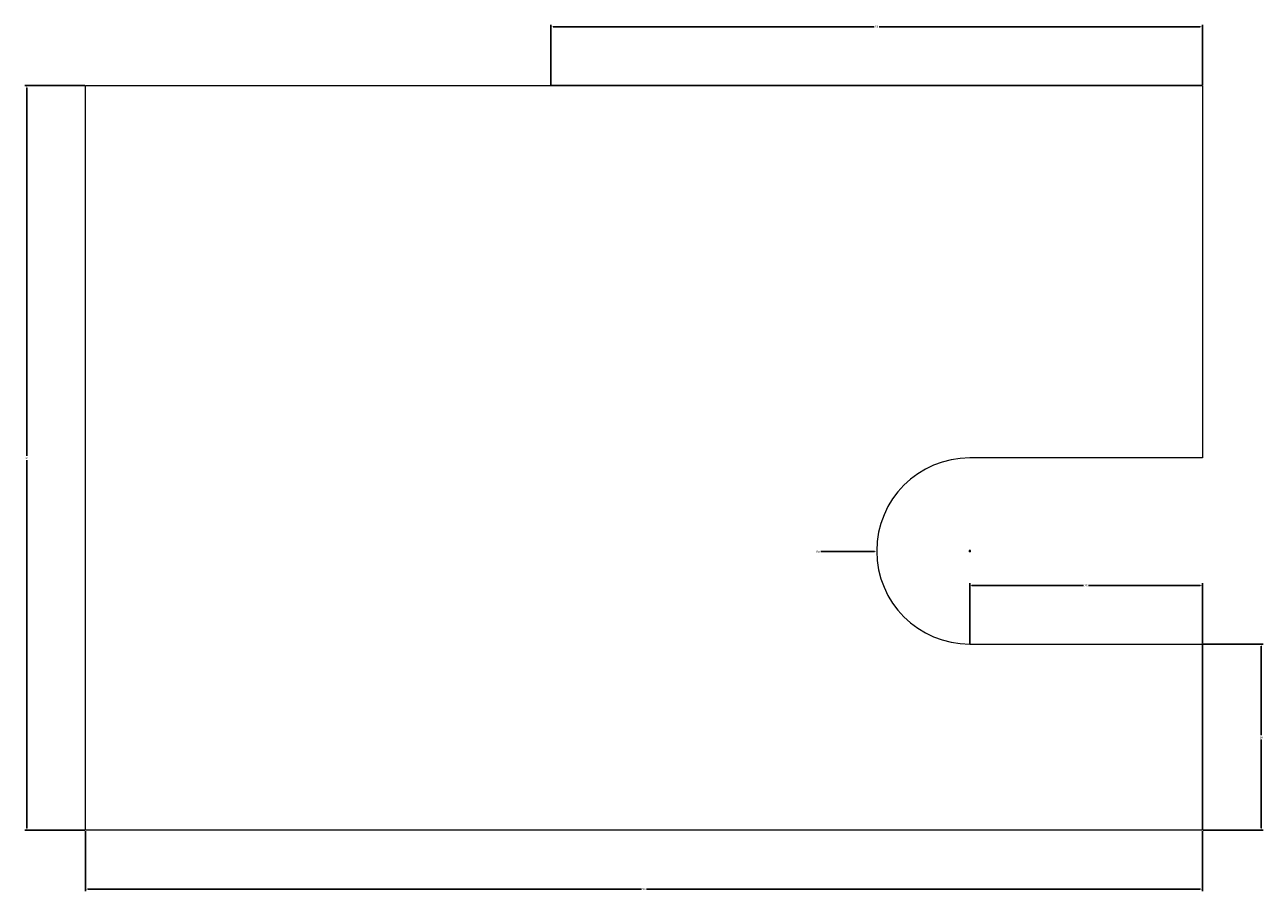
# Model space of a CAD drawing. Units: millimetres. Extents: x -4 to 2856, y -2 to 1373.
# Tile 3 of 3: x 2749 to 2856, y 1175 to 1249. Entities that reach past the tile are written whole.
import ezdxf

# ---------------------------------------------------------------- set-up
doc = ezdxf.new("R2010")
doc.units = ezdxf.units.MM
doc.layers.add('M-CONS', color=8, linetype='Continuous', lineweight=18)
doc.layers.add('M-DIMS', color=2, linetype='Continuous', lineweight=18)
doc.styles.get("Standard").update_dxf_attribs({"font": 'arial.ttf'})
doc.dimstyles.get("Standard").update_dxf_attribs({"dimtxt": 0.18, "dimasz": 0.18, "dimexe": 0.18, "dimexo": 0.0625, "dimgap": 0.09, "dimtad": 0, "dimtih": 1, "dimtoh": 1, "dimdec": 4, "dimzin": 0, "dimdsep": 46, "dimtxsty": 'Standard', "dimcen": 0.09, "dimadec": 0, "dimazin": 0, "dimtfac": 1, "dimtdec": 4, "dimtofl": 0, "dimtmove": 0, "dimatfit": 3, "dimfxl": 1, "dimtolj": 1, "dimtzin": 0, "dimarcsym": 0})

# ---------------------------------------------------------------- blocks, each defined once
blk = doc.blocks.new('*D1')
at = {"layer": 'Defpoints', "color": 0, "transparency": 16777216}
for p in [(2850.61, 1249.28), (2794.61, 1244.23), (2850.61, 1244.23)]:
    blk.add_point(p, dxfattribs=at)
at = {"layer": 'M-DIMS', "color": 0, "lineweight": -2, "transparency": 16777216}
for p, q in [((2794.61, 1244.29), (2794.61, 1249.46)), ((2794.79, 1249.28), (2822.39, 1249.28)), ((2850.43, 1249.28), (2822.83, 1249.28)), ((2850.61, 1244.29), (2850.61, 1249.46))]:
    blk.add_line(p, q, dxfattribs=at)
at = {"layer": 'M-DIMS', "color": 0, "transparency": 16777216}
for points in [[(2794.79, 1249.31), (2794.79, 1249.25), (2794.61, 1249.28)], [(2850.43, 1249.31), (2850.43, 1249.25), (2850.61, 1249.28)]]:
    blk.add_solid(points, dxfattribs=at)
at = {"layer": 'M-DIMS', "color": 0, "transparency": 16777216, "insert": (2822.61, 1249.28), "char_height": 0.18, "attachment_point": 5}
blk.add_mtext('\\A1;56', dxfattribs=at)
blk = doc.blocks.new('*D2')
at = {"layer": 'Defpoints', "color": 0, "transparency": 16777216}
for p in [(2754.61, 1180.23), (2850.61, 1180.23), (2850.61, 1175.18)]:
    blk.add_point(p, dxfattribs=at)
at = {"layer": 'M-DIMS', "color": 0, "lineweight": -2, "transparency": 16777216}
for p, q in [((2754.61, 1180.16), (2754.61, 1175)), ((2850.61, 1180.16), (2850.61, 1175)), ((2754.79, 1175.18), (2802.39, 1175.18)), ((2850.43, 1175.18), (2802.83, 1175.18))]:
    blk.add_line(p, q, dxfattribs=at)
at = {"layer": 'M-DIMS', "color": 0, "transparency": 16777216}
for points in [[(2754.79, 1175.21), (2754.79, 1175.15), (2754.61, 1175.18)], [(2850.43, 1175.21), (2850.43, 1175.15), (2850.61, 1175.18)]]:
    blk.add_solid(points, dxfattribs=at)
at = {"layer": 'M-DIMS', "color": 0, "transparency": 16777216, "insert": (2802.61, 1175.18), "char_height": 0.18, "attachment_point": 5}
blk.add_mtext('\\A1;96', dxfattribs=at)
blk = doc.blocks.new('*D3')
at = {"layer": 'Defpoints', "color": 0, "transparency": 16777216}
for p in [(2749.56, 1244.23), (2754.61, 1244.23), (2754.61, 1180.23)]:
    blk.add_point(p, dxfattribs=at)
at = {"layer": 'M-DIMS', "color": 0, "lineweight": -2, "transparency": 16777216}
for p, q in [((2754.54, 1244.23), (2749.38, 1244.23)), ((2749.56, 1244.05), (2749.56, 1212.41)), ((2749.56, 1180.41), (2749.56, 1212.04)), ((2754.54, 1180.23), (2749.38, 1180.23))]:
    blk.add_line(p, q, dxfattribs=at)
at = {"layer": 'M-DIMS', "color": 0, "transparency": 16777216}
for points in [[(2749.53, 1244.05), (2749.59, 1244.05), (2749.56, 1244.23)], [(2749.53, 1180.41), (2749.59, 1180.41), (2749.56, 1180.23)]]:
    blk.add_solid(points, dxfattribs=at)
at = {"layer": 'M-DIMS', "color": 0, "transparency": 16777216, "insert": (2749.56, 1212.23), "char_height": 0.18, "attachment_point": 5}
blk.add_mtext('\\A1;64', dxfattribs=at)
blk = doc.blocks.new('*D4')
at = {"layer": 'Defpoints', "color": 0, "transparency": 16777216}
for p in [(2850.61, 1201.28), (2830.61, 1196.23), (2850.61, 1196.23)]:
    blk.add_point(p, dxfattribs=at)
at = {"layer": 'M-DIMS', "color": 0, "lineweight": -2, "transparency": 16777216}
for p, q in [((2830.61, 1196.29), (2830.61, 1201.46)), ((2830.79, 1201.28), (2840.39, 1201.28)), ((2850.43, 1201.28), (2840.83, 1201.28)), ((2850.61, 1196.29), (2850.61, 1201.46))]:
    blk.add_line(p, q, dxfattribs=at)
at = {"layer": 'M-DIMS', "color": 0, "transparency": 16777216}
for points in [[(2830.79, 1201.31), (2830.79, 1201.25), (2830.61, 1201.28)], [(2850.43, 1201.31), (2850.43, 1201.25), (2850.61, 1201.28)]]:
    blk.add_solid(points, dxfattribs=at)
at = {"layer": 'M-DIMS', "color": 0, "transparency": 16777216, "insert": (2840.61, 1201.28), "char_height": 0.18, "attachment_point": 5}
blk.add_mtext('\\A1;20', dxfattribs=at)
blk = doc.blocks.new('*D5')
at = {"layer": 'Defpoints', "color": 0, "transparency": 16777216}
for p in [(2850.61, 1196.23), (2855.66, 1196.23), (2850.61, 1180.23)]:
    blk.add_point(p, dxfattribs=at)
at = {"layer": 'M-DIMS', "color": 0, "lineweight": -2, "transparency": 16777216}
for p, q in [((2850.67, 1196.23), (2855.84, 1196.23)), ((2855.66, 1196.05), (2855.66, 1188.41)), ((2855.66, 1180.41), (2855.66, 1188.04)), ((2850.67, 1180.23), (2855.84, 1180.23))]:
    blk.add_line(p, q, dxfattribs=at)
at = {"layer": 'M-DIMS', "color": 0, "transparency": 16777216}
for points in [[(2855.63, 1196.05), (2855.69, 1196.05), (2855.66, 1196.23)], [(2855.63, 1180.41), (2855.69, 1180.41), (2855.66, 1180.23)]]:
    blk.add_solid(points, dxfattribs=at)
at = {"layer": 'M-DIMS', "color": 0, "transparency": 16777216, "insert": (2855.66, 1188.23), "char_height": 0.18, "attachment_point": 5}
blk.add_mtext('\\A1;16', dxfattribs=at)
blk = doc.blocks.new('*D10')
at = {"layer": 'Defpoints', "color": 0, "transparency": 16777216}
for p in [(2822.61, 1204.2), (2830.61, 1204.23)]:
    blk.add_point(p, dxfattribs=at)
at = {"layer": 'M-DIMS', "color": 0, "lineweight": -2, "transparency": 16777216}
for p, q in [((2817.81, 1204.18), (2822.43, 1204.2)), ((2830.52, 1204.23), (2830.7, 1204.23)), ((2830.61, 1204.14), (2830.61, 1204.32))]:
    blk.add_line(p, q, dxfattribs=at)
at = {"layer": 'M-DIMS', "color": 0, "transparency": 16777216}
blk.add_solid([(2822.43, 1204.23), (2822.43, 1204.17), (2822.61, 1204.2)], dxfattribs=at)
at = {"layer": 'M-DIMS', "color": 0, "transparency": 16777216, "insert": (2817.57, 1204.18), "char_height": 0.18, "attachment_point": 5}
blk.add_mtext('\\A1;R8', dxfattribs=at)

msp = doc.modelspace()

# ---------------------------------------------------------------- linework, layer by layer
at = {"layer": 'M-CONS'}
msp.add_lwpolyline([(2850.61, 1180.23), (2754.61, 1180.23), (2754.61, 1244.23), (2850.61, 1244.23), (2850.61, 1212.23), (2830.61, 1212.23, 1), (2830.61, 1196.23), (2850.61, 1196.23), (2850.61, 1180.23), (2850.61, 1196.23)], format="xyb", dxfattribs=at)
at = {"layer": 'M-CONS', "extrusion": (0, -1, 0), "elevation": -1244.23}
msp.add_lwpolyline([(2794.61, 16), (2850.61, 16), (2794.61, 44)], close=True, dxfattribs=at)

# ---------------------------------------------------------------- dimensions: what is measured, and where the dimension line sits
at = {"layer": 'M-DIMS'}
for base, p1, p2, picture, middle in [((2850.61, 1249.28), (2794.61, 1244.23), (2850.61, 1244.23), '*D1', (2822.61, 1249.28)), ((2850.61, 1201.28), (2830.61, 1196.23), (2850.61, 1196.23), '*D4', (2840.61, 1201.28)), ((2850.61, 1175.18), (2754.61, 1180.23), (2850.61, 1180.23), '*D2', (2802.61, 1175.18))]:
    dim = msp.add_linear_dim(base=base, p1=p1, p2=p2, dimstyle='Standard', override={"dimdec": 0, "dimlfac": 1, "dimrnd": 0, "dimzin": 0, "dimdsep": 46, "dimlunit": 2}, dxfattribs=at)
    dim.commit()
    dim.dimension.update_dxf_attribs({"geometry": picture, "text_midpoint": middle})
for base, p1, p2, picture, middle in [((2749.56, 1244.23), (2754.61, 1180.23), (2754.61, 1244.23), '*D3', (2749.56, 1212.23)), ((2855.66, 1196.23), (2850.61, 1180.23), (2850.61, 1196.23), '*D5', (2855.66, 1188.23))]:
    dim = msp.add_linear_dim(base=base, p1=p1, p2=p2, angle=90, dimstyle='Standard', override={"dimdec": 0, "dimlfac": 1, "dimrnd": 0, "dimzin": 0, "dimdsep": 46, "dimlunit": 2}, dxfattribs=at)
    dim.commit()
    dim.dimension.update_dxf_attribs({"geometry": picture, "text_midpoint": middle})
dim = msp.add_radius_dim(center=(2830.61, 1204.23), mpoint=(2822.61, 1204.2), dimstyle='Standard', override={"dimdec": 0, "dimlfac": 1, "dimrnd": 0, "dimzin": 0, "dimdsep": 46, "dimlunit": 2}, dxfattribs=at)
dim.commit()
dim.dimension.update_dxf_attribs({"geometry": '*D10', "text_midpoint": (2817.81, 1204.18), "dimtype": 164})

doc.saveas('drawing.dxf')
